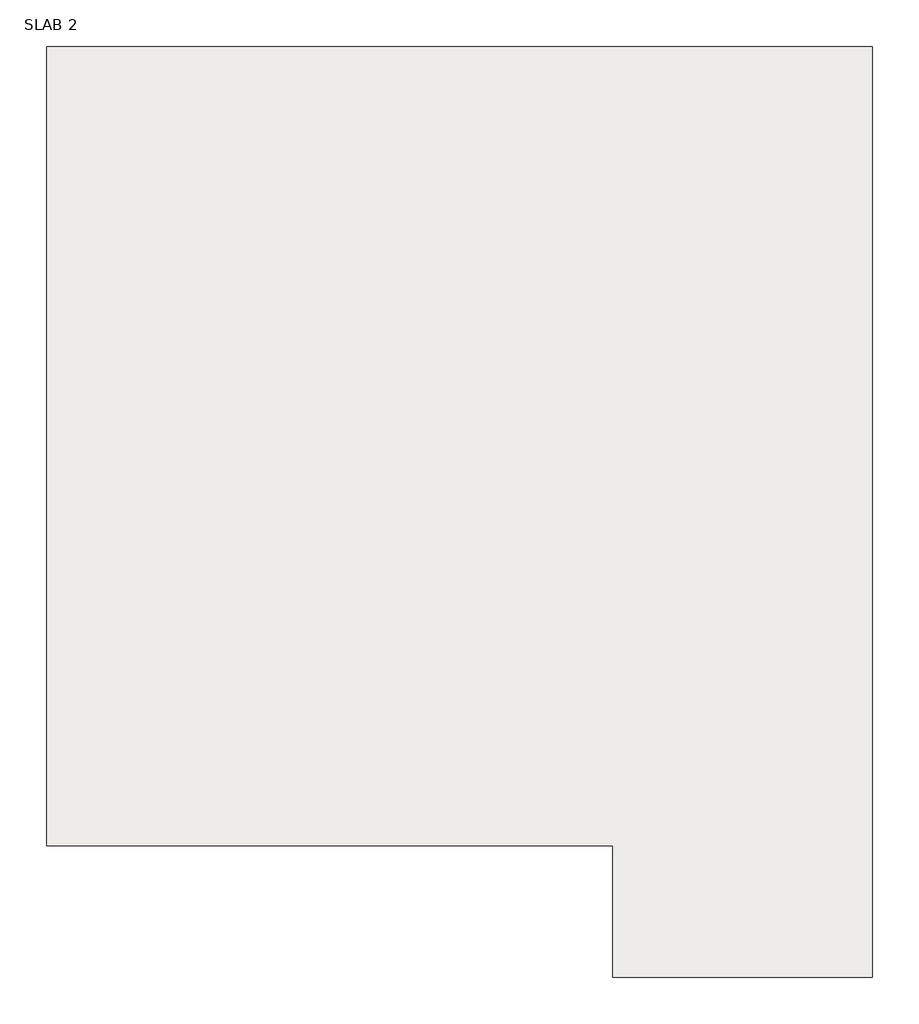
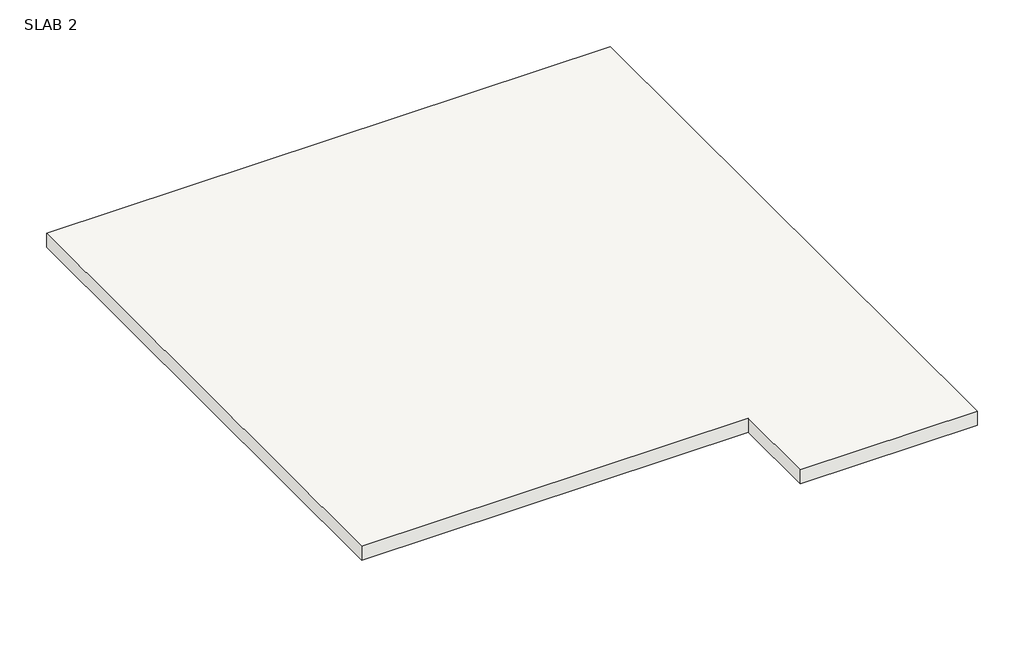
# One storey: 1 slab.
"""IFC4 building model written with IfcOpenShell, lengths in millimetres."""

from ifc_helpers import new_model, si_unit, frame, origin, place, context, project, spatial, polyline, outline, extrude, element, save

model = new_model("IFC4")

# Units and contexts
model_context = context("Model", 3, world=origin())
ifc_project = project(units=[si_unit("LENGTHUNIT", "METRE", prefix="MILLI")], contexts=[model_context])

# Site, building, storey
site = spatial("IfcSite", under=ifc_project)
building = spatial("IfcBuilding", under=site)
storey = spatial("IfcBuildingStorey", under=building, Name="SLAB 2", Elevation=10363.2)

# Slab
placement = place(None, origin())
element("IfcSlab", 1, ObjectType="Generic - 12\"", at=placement, inside=storey, context=model_context, shape_type="SweptSolid", body=[
    extrude(outline(polyline([(3739.3918749, 13083.8953049), (3739.3918749, 53.6953049), (107.1918749, 53.6953049), (107.1918749, 1895.1953049), (-7817.6081251, 1895.1953049), (-7817.6081251, 13083.8953049), (3739.3918749, 13083.8953049)])), frame((0.0, 0.0, 10058.4), z_axis=(0.0, 0.0, 1.0), x_axis=(1.0, 0.0, 0.0)), (0.0, 0.0, 1.0), 304.8),
])

save(model, "model.ifc")

# Revit data of these elements
# Type "Generic - 12\""
#   Assembly Code = "B1010"
#   Function = 0
#   Layers, outside or top first: 1' - 0" no material (function 1)
# Element 1 (IfcSlab, "Generic - 12\"")
#   Height Offset From Level = 0' - 0"
#   Phase Created = New Construction
#   Materials on its faces: "Default Floor", "Acoustic Ceiling Tile 24 x 24"
# Materials
#   "Default Floor": colour RGB 128 128 128, transparency 0, Cost = 0
#   "Acoustic Ceiling Tile 24 x 24": class "Generic", colour RGB 232 232 232, transparency 0, Description = "Acoustic Ceiling Tile 24 x 24", Cost = 0
